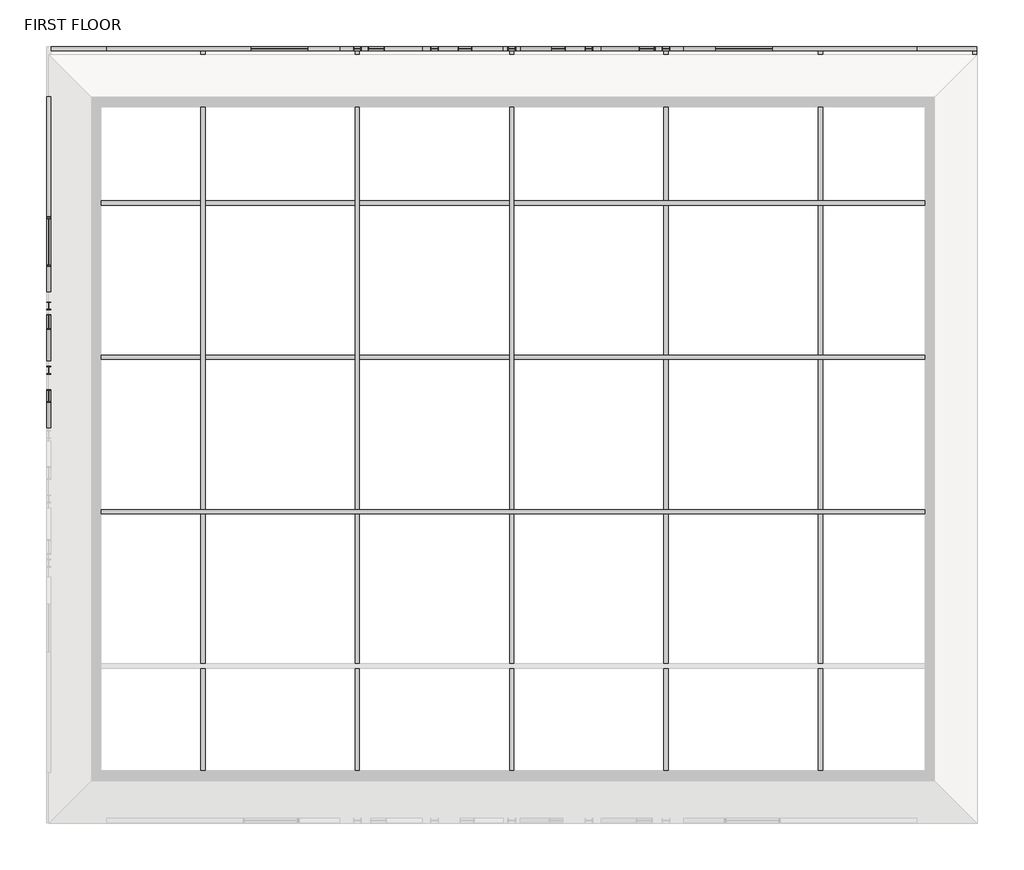
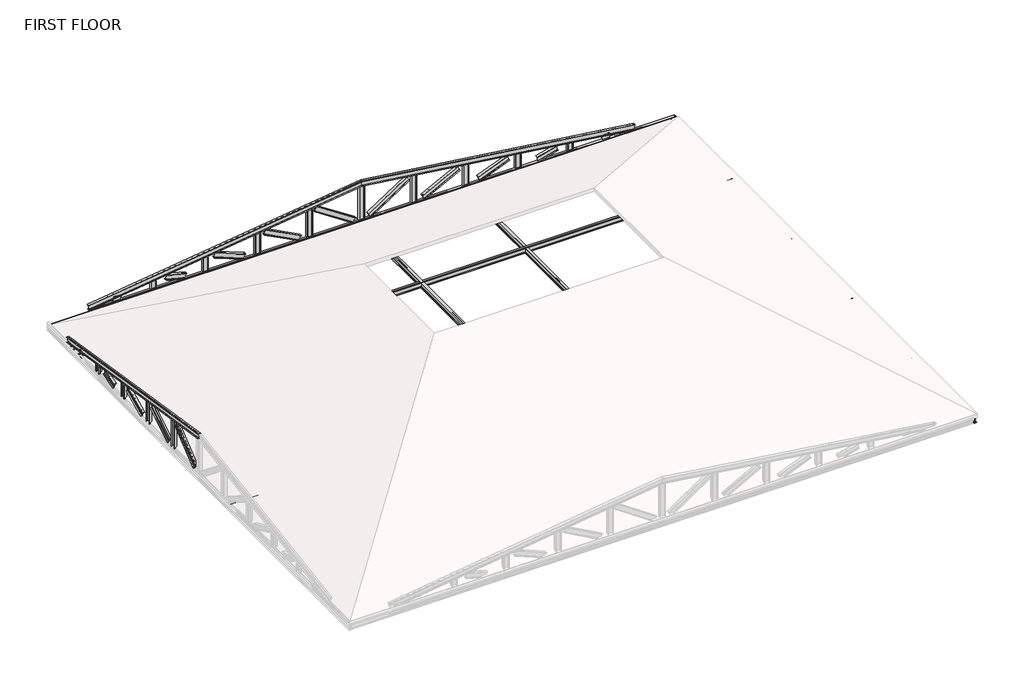
# One storey, part 2 of 2: 45 beams.
"""IFC4 building model written with IfcOpenShell, lengths in millimetres."""

from ifc_helpers import new_model, si_unit, frame, origin, place, context, project, spatial, polyline, circle_curve, ellipse_curve, transform, mapped, element, save
from ifc_brep_helpers import plane_surface, revolved_surface, advanced_brep
from components import ub_universal_beams_ub305x165x40_be890a2c, ub_universal_beams_ub305x165x40_a59d1a35, ub_universal_beams_ub305x165x40_0aabe8ba, ub_universal_beams_ub305x165x40_d04475ed, ub_universal_beams_ub305x165x40_f264fe8a, ub_universal_beams_ub305x165x40_2f8ff02f, ub_universal_beams_ub305x165x40_4bff7ce7, ub_universal_beams_ub305x165x40_d5ce0422, ub_universal_beams_ub305x165x40_0af343aa, ub_universal_beams_ub305x165x40_6c2df09e, ub_universal_beams_ub305x165x40_9aefeb6a, ub_universal_beams_ub305x165x40_8fd3c0bc, ub_universal_beams_ub305x165x40_dcb3c2ea, ub_universal_beams_ub305x165x40_5cbd381f, ub_universal_beams_ub305x165x40_28de461c, ub_universal_beams_ub305x165x40_2a071682, ub_universal_beams_ub305x165x40_a83b25bc, ub_universal_beams_ub305x165x40_c2ddfea9, ub_universal_beams_ub305x165x40_890a58b8, ub_universal_beams_ub305x165x40_8a566974, ub_universal_beams_ub305x165x40_7abb9ae2, ub_universal_beams_ub305x165x40_eb09afc0, ub_universal_beams_ub305x165x40_07ff8ca2, ub_universal_beams_ub305x165x40_bc9e57b7, ub_universal_beams_ub305x165x40_1f6689ec, ub_universal_beams_ub305x165x40_ea68f55e, ub_universal_beams_ub305x165x40_862170f4, ub_universal_beams_ub305x165x40_9b118c67, ub_universal_beams_ub305x165x40_fca44d3c, ub_universal_beams_ub305x165x40_5ea05da3

model = new_model("IFC4")

# Units and contexts
model_context = context("Model", 3, world=origin())
ifc_project = project(units=[si_unit("LENGTHUNIT", "METRE", prefix="MILLI")], contexts=[model_context])

# Site, building, storey
site = spatial("IfcSite", under=ifc_project)
building = spatial("IfcBuilding", under=site)
storey = spatial("IfcBuildingStorey", under=building, Name="FIRST FLOOR", Elevation=2454.6695361)

# Beams
placement = place(None, origin())
element("IfcBeam", 1, ObjectType="UB-Universal Beams : UB305x165x40", at=placement, inside=storey, context=model_context, shape_type="AdvancedBrep", body=[
    advanced_brep(
    [(-16297.3812503, 24370.7691735, 2618.146307), (-16296.0540475, 24370.7691735, 2608.033022), (-16296.0540475, 24205.7691735, 2608.033022), (-16297.3812503, 24205.7691735, 2618.146307), (-16297.3812503, 24276.3691735, 2618.146307), (-16298.5392997, 24285.2691735, 2626.9706439), (-16333.0465713, 24285.2691735, 2889.9160531), (-16334.2046207, 24276.3691735, 2898.7403899), (-16334.2046207, 24205.7691735, 2898.7403899), (-16335.5318235, 24205.7691735, 2908.8536749), (-16335.5318235, 24370.7691735, 2908.8536749), (-16334.2046207, 24370.7691735, 2898.7403899), (-16334.2046207, 24300.1691735, 2898.7403899), (-16333.0465713, 24291.2691735, 2889.9160531), (-16298.5392997, 24291.2691735, 2626.9706439), (-16297.3812503, 24300.1691735, 2618.146307), (-342.5493858, 24300.1691735, 4711.9562629), (-342.5493858, 24370.7691735, 4711.9562629), (-342.5493858, 24291.2691735, 4720.9325748), (-342.5493858, 24291.2691735, 4988.4064973), (-342.5493858, 24300.1691735, 4997.3828092), (-342.5493858, 24370.7691735, 4997.3828092), (-342.5493858, 24370.7691735, 5007.6702678), (-342.5493858, 24205.7691735, 5007.6702678), (-342.5493858, 24205.7691735, 4997.3828092), (-342.5493858, 24276.3691735, 4997.3828092), (-342.5493858, 24285.2691735, 4988.4064973), (-342.5493858, 24285.2691735, 4720.9325748), (-342.5493858, 24276.3691735, 4711.9562629), (-342.5493858, 24205.7691735, 4711.9562629), (-342.5493858, 24205.7691735, 4701.6688044), (-342.5493858, 24370.7691735, 4701.6688044)],
    [
        (0, 1),
        (1, 2),
        (2, 3),
        (3, 4),
        (4, 5, circle_curve(frame((-16298.5392997, 24276.3691735, 2626.9706439), z_axis=(0.9914985263311615, 0.0, 0.13011791684135987), x_axis=(0.0, -1.0, 0.0)), 8.9)),
        (5, 6),
        (6, 7, circle_curve(frame((-16333.0465713, 24276.3691735, 2889.9160531), z_axis=(0.9914985263311615, 0.0, 0.13011791684135987), x_axis=(0.0, -1.0, 0.0)), 8.9)),
        (7, 8),
        (8, 9),
        (9, 10),
        (10, 11),
        (11, 12),
        (12, 13, circle_curve(frame((-16333.0465713, 24300.1691735, 2889.9160531), z_axis=(0.9914985263311615, 0.0, 0.13011791684135987), x_axis=(0.0, -1.0, 0.0)), 8.9)),
        (13, 14),
        (14, 15, circle_curve(frame((-16298.5392997, 24300.1691735, 2626.9706439), z_axis=(0.9914985263311615, 0.0, 0.13011791684135987), x_axis=(0.0, -1.0, 0.0)), 8.9)),
        (15, 0),
        (16, 17),
        (17, 0),
        (15, 16),
        (18, 16, ellipse_curve(frame((-342.5493858, 24300.1691735, 4720.9325748), z_axis=(1.0, 0.0, 0.0), x_axis=(0.0, 0.0, -0.9999999999999999)), 8.9763119, 8.9)),
        (14, 18),
        (19, 18),
        (13, 19),
        (20, 19, ellipse_curve(frame((-342.5493858, 24300.1691735, 4988.4064973), z_axis=(1.0, 0.0, 0.0), x_axis=(0.0, 0.0, -0.9999999999999999)), 8.9763119, 8.9)),
        (12, 20),
        (21, 20),
        (11, 21),
        (22, 21),
        (10, 22),
        (23, 22),
        (9, 23),
        (24, 23),
        (8, 24),
        (25, 24),
        (7, 25),
        (26, 25, ellipse_curve(frame((-342.5493858, 24276.3691735, 4988.4064973), z_axis=(1.0, 0.0, 0.0), x_axis=(0.0, 0.0, -0.9999999999999999)), 8.9763119, 8.9)),
        (6, 26),
        (27, 26),
        (5, 27),
        (28, 27, ellipse_curve(frame((-342.5493858, 24276.3691735, 4720.9325748), z_axis=(1.0, 0.0, 0.0), x_axis=(0.0, 0.0, -0.9999999999999999)), 8.9763119, 8.9)),
        (4, 28),
        (29, 28),
        (3, 29),
        (30, 29),
        (2, 30),
        (31, 30),
        (1, 31),
        (17, 31),
    ],
    [
        plane_surface(frame((-16315.7929355, 24288.2691735, 2758.4433485), z_axis=(-0.9914985263311615, 0.0, -0.13011791684135987), x_axis=(-0.13011791684135987, 0.0, 0.9914985263311615))),
        plane_surface(frame((-324.1416914, 24370.7691735, 4714.3719709), z_axis=(-0.13011791684135987, 0.0, 0.9914985263311615), x_axis=(-0.9914985263311615, 0.0, -0.13011791684135987))),
        revolved_surface(polyline([(-16298.5392997612, 24291.269173499997, 2626.970643894329), (-341.39133634520147, 24291.269173499997, 4721.084549854435)]), (-325.2997408, 24300.1691735, 4723.1963078), (-0.9914985263311615, 0.0, -0.13011791684135987)),
        plane_surface(frame((-325.2997408, 24291.2691735, 4723.1963078), z_axis=(0.0, 1.0, 0.0), x_axis=(-0.9914985263311615, 0.0, -0.13011791684135987))),
        revolved_surface(polyline([(-16333.046571287405, 24291.269173499997, 2889.9160530040135), (-341.3913363366006, 24291.269173499997, 4988.558472288897)]), (-359.8070124, 24300.1691735, 4986.1417169), (-0.9914985263311615, 0.0, -0.13011791684135987)),
        plane_surface(frame((-360.9650618, 24300.1691735, 4994.9660538), z_axis=(0.13011791684135987, 0.0, -0.9914985263311615), x_axis=(-0.9914985263311615, 0.0, -0.13011791684135987))),
        plane_surface(frame((-360.9650618, 24370.7691735, 4994.9660538), z_axis=(0.0, 1.0, 0.0), x_axis=(-0.9914985263311615, 0.0, -0.13011791684135987))),
        plane_surface(frame((-362.2922646, 24370.7691735, 5005.0793388), z_axis=(-0.13011791684135987, 0.0, 0.9914985263311615), x_axis=(-0.9914985263311615, 0.0, -0.13011791684135987))),
        plane_surface(frame((-362.2922646, 24205.7691735, 5005.0793388), z_axis=(0.0, -1.0, 0.0), x_axis=(-0.9914985263311615, 0.0, -0.13011791684135987))),
        plane_surface(frame((-360.9650618, 24205.7691735, 4994.9660538), z_axis=(0.13011791684135987, 0.0, -0.9914985263311615), x_axis=(-0.9914985263311615, 0.0, -0.13011791684135987))),
        revolved_surface(polyline([(-16333.046571287405, 24267.469173499998, 2889.9160530040135), (-341.3913363366006, 24267.469173499998, 4988.558472288897)]), (-359.8070124, 24276.3691735, 4986.1417169), (-0.9914985263311615, 0.0, -0.13011791684135987)),
        plane_surface(frame((-359.8070124, 24285.2691735, 4986.1417169), z_axis=(0.0, -1.0, 0.0), x_axis=(-0.9914985263311615, 0.0, -0.13011791684135987))),
        revolved_surface(polyline([(-16298.5392997612, 24267.469173499998, 2626.970643894329), (-341.39133634520147, 24267.469173499998, 4721.084549854435)]), (-325.2997408, 24276.3691735, 4723.1963078), (-0.9914985263311615, 0.0, -0.13011791684135987)),
        plane_surface(frame((-324.1416914, 24276.3691735, 4714.3719709), z_axis=(-0.13011791684135987, 0.0, 0.9914985263311615), x_axis=(-0.9914985263311615, 0.0, -0.13011791684135987))),
        plane_surface(frame((-324.1416914, 24205.7691735, 4714.3719709), z_axis=(0.0, -1.0, 0.0), x_axis=(-0.9914985263311615, 0.0, -0.13011791684135987))),
        plane_surface(frame((-322.8144886, 24205.7691735, 4704.2586859), z_axis=(0.13011791684135987, 0.0, -0.9914985263311615), x_axis=(-0.9914985263311615, 0.0, -0.13011791684135987))),
        plane_surface(frame((-322.8144886, 24370.7691735, 4704.2586859), z_axis=(0.0, 1.0, 0.0), x_axis=(-0.9914985263311615, 0.0, -0.13011791684135987))),
        plane_surface(frame((-342.5493858, 24288.2691735, 5007.6702678), z_axis=(1.0, 0.0, 0.0), x_axis=(0.0, -1.0, 0.0))),
    ],
    [
        (0, [[1, 2, 3, 4, 5, 6, 7, 8, 9, 10, 11, 12, 13, 14, 15, 16]]),
        (1, [[17, 18, -16, 19]]),
        (2, [[20, -19, -15, 21]]),
        (3, [[22, -21, -14, 23]]),
        (4, [[24, -23, -13, 25]]),
        (5, [[26, -25, -12, 27]]),
        (6, [[28, -27, -11, 29]]),
        (7, [[30, -29, -10, 31]]),
        (8, [[32, -31, -9, 33]]),
        (9, [[34, -33, -8, 35]]),
        (10, [[36, -35, -7, 37]]),
        (11, [[38, -37, -6, 39]]),
        (12, [[40, -39, -5, 41]]),
        (13, [[42, -41, -4, 43]]),
        (14, [[44, -43, -3, 45]]),
        (15, [[46, -45, -2, 47]]),
        (16, [[48, -47, -1, -18]]),
        (17, [[-17, -20, -22, -24, -26, -28, -30, -32, -34, -36, -38, -40, -42, -44, -46, -48]]),
    ],
),
])
element("IfcBeam", 2, ObjectType="UB-Universal Beams : UB305x165x40", at=placement, inside=storey, context=model_context, shape_type="AdvancedBrep", body=[
    advanced_brep(
    [(15612.2824786, 24370.7691735, 2618.146307), (15612.2824786, 24300.1691735, 2618.146307), (15613.4405281, 24291.2691735, 2626.9706439), (15647.9477996, 24291.2691735, 2889.9160531), (15649.1058491, 24300.1691735, 2898.7403899), (15649.1058491, 24370.7691735, 2898.7403899), (15650.4330518, 24370.7691735, 2908.8536749), (15650.4330518, 24205.7691735, 2908.8536749), (15649.1058491, 24205.7691735, 2898.7403899), (15649.1058491, 24276.3691735, 2898.7403899), (15647.9477996, 24285.2691735, 2889.9160531), (15613.4405281, 24285.2691735, 2626.9706439), (15612.2824786, 24276.3691735, 2618.146307), (15612.2824786, 24205.7691735, 2618.146307), (15610.9552758, 24205.7691735, 2608.033022), (15610.9552758, 24370.7691735, 2608.033022), (-342.5493858, 24370.7691735, 4711.9562629), (-342.5493858, 24300.1691735, 4711.9562629), (-342.5493858, 24291.2691735, 4720.9325748), (-342.5493858, 24291.2691735, 4988.4064973), (-342.5493858, 24300.1691735, 4997.3828092), (-342.5493858, 24370.7691735, 4997.3828092), (-342.5493858, 24370.7691735, 5007.6702678), (-342.5493858, 24205.7691735, 5007.6702678), (-342.5493858, 24205.7691735, 4997.3828092), (-342.5493858, 24276.3691735, 4997.3828092), (-342.5493858, 24285.2691735, 4988.4064973), (-342.5493858, 24285.2691735, 4720.9325748), (-342.5493858, 24276.3691735, 4711.9562629), (-342.5493858, 24205.7691735, 4711.9562629), (-342.5493858, 24205.7691735, 4701.6688044), (-342.5493858, 24370.7691735, 4701.6688044)],
    [
        (0, 1),
        (1, 2, circle_curve(frame((15613.4405281, 24300.1691735, 2626.9706439), z_axis=(-0.9914985263311615, 0.0, 0.13011791684135987), x_axis=(0.0, -1.0, 0.0)), 8.9)),
        (2, 3),
        (3, 4, circle_curve(frame((15647.9477996, 24300.1691735, 2889.9160531), z_axis=(-0.9914985263311615, 0.0, 0.13011791684135987), x_axis=(0.0, -1.0, 0.0)), 8.9)),
        (4, 5),
        (5, 6),
        (6, 7),
        (7, 8),
        (8, 9),
        (9, 10, circle_curve(frame((15647.9477996, 24276.3691735, 2889.9160531), z_axis=(-0.9914985263311615, 0.0, 0.13011791684135987), x_axis=(0.0, -1.0, 0.0)), 8.9)),
        (10, 11),
        (11, 12, circle_curve(frame((15613.4405281, 24276.3691735, 2626.9706439), z_axis=(-0.9914985263311615, 0.0, 0.13011791684135987), x_axis=(0.0, -1.0, 0.0)), 8.9)),
        (12, 13),
        (13, 14),
        (14, 15),
        (15, 0),
        (0, 16),
        (16, 17),
        (17, 1),
        (17, 18, ellipse_curve(frame((-342.5493858, 24300.1691735, 4720.9325748), z_axis=(-1.0, 0.0, 0.0), x_axis=(0.0, 0.0, 1.0)), 8.9763119, 8.9)),
        (18, 2),
        (18, 19),
        (19, 3),
        (19, 20, ellipse_curve(frame((-342.5493858, 24300.1691735, 4988.4064973), z_axis=(-1.0, 0.0, 0.0), x_axis=(0.0, 0.0, 1.0)), 8.9763119, 8.9)),
        (20, 4),
        (20, 21),
        (21, 5),
        (21, 22),
        (22, 6),
        (22, 23),
        (23, 7),
        (23, 24),
        (24, 8),
        (24, 25),
        (25, 9),
        (25, 26, ellipse_curve(frame((-342.5493858, 24276.3691735, 4988.4064973), z_axis=(-1.0, 0.0, 0.0), x_axis=(0.0, 0.0, 1.0)), 8.9763119, 8.9)),
        (26, 10),
        (26, 27),
        (27, 11),
        (27, 28, ellipse_curve(frame((-342.5493858, 24276.3691735, 4720.9325748), z_axis=(-1.0, 0.0, 0.0), x_axis=(0.0, 0.0, 1.0)), 8.9763119, 8.9)),
        (28, 12),
        (28, 29),
        (29, 13),
        (29, 30),
        (30, 14),
        (30, 31),
        (31, 15),
        (31, 16),
    ],
    [
        plane_surface(frame((15630.6941638, 24288.2691735, 2758.4433485), z_axis=(0.9914985263311615, 0.0, -0.13011791684135987), x_axis=(0.13011791684135987, 0.0, 0.9914985263311615))),
        plane_surface(frame((15612.2824786, 24370.7691735, 2618.146307), z_axis=(0.13011791684135987, 0.0, 0.9914985263311615), x_axis=(-0.9914985263311615, 0.0, 0.13011791684135987))),
        revolved_surface(polyline([(-343.70743525510625, 24291.269173499997, 4721.084549852116), (15613.4405281, 24291.269173499997, 2626.9706439)]), (15613.4405281, 24300.1691735, 2626.9706439), (-0.9914985263311615, 0.0, 0.13011791684135987)),
        plane_surface(frame((15613.4405281, 24291.2691735, 2626.9706439), z_axis=(0.0, 1.0, 0.0), x_axis=(-0.9914985263311615, 0.0, 0.13011791684135987))),
        revolved_surface(polyline([(-343.707435252496, 24291.269173499997, 4988.558472371982), (15647.947799650316, 24291.269173499997, 2889.9160530933973)]), (15647.9477996, 24300.1691735, 2889.9160531), (-0.9914985263311615, 0.0, 0.13011791684135987)),
        plane_surface(frame((15649.1058491, 24300.1691735, 2898.7403899), z_axis=(-0.13011791684135987, 0.0, -0.9914985263311615), x_axis=(-0.9914985263311615, 0.0, 0.13011791684135987))),
        plane_surface(frame((15649.1058491, 24370.7691735, 2898.7403899), z_axis=(0.0, 1.0, 0.0), x_axis=(-0.9914985263311615, 0.0, 0.13011791684135987))),
        plane_surface(frame((15650.4330518, 24370.7691735, 2908.8536749), z_axis=(0.13011791684135987, 0.0, 0.9914985263311615), x_axis=(-0.9914985263311615, 0.0, 0.13011791684135987))),
        plane_surface(frame((15650.4330518, 24205.7691735, 2908.8536749), z_axis=(0.0, -1.0, 0.0), x_axis=(-0.9914985263311615, 0.0, 0.13011791684135987))),
        plane_surface(frame((15649.1058491, 24205.7691735, 2898.7403899), z_axis=(-0.13011791684135987, 0.0, -0.9914985263311615), x_axis=(-0.9914985263311615, 0.0, 0.13011791684135987))),
        revolved_surface(polyline([(-343.707435252496, 24267.469173499998, 4988.558472371982), (15647.947799650316, 24267.469173499998, 2889.9160530933973)]), (15647.9477996, 24276.3691735, 2889.9160531), (-0.9914985263311615, 0.0, 0.13011791684135987)),
        plane_surface(frame((15647.9477996, 24285.2691735, 2889.9160531), z_axis=(0.0, -1.0, 0.0), x_axis=(-0.9914985263311615, 0.0, 0.13011791684135987))),
        revolved_surface(polyline([(-343.70743525510625, 24267.469173499998, 4721.084549852116), (15613.4405281, 24267.469173499998, 2626.9706439)]), (15613.4405281, 24276.3691735, 2626.9706439), (-0.9914985263311615, 0.0, 0.13011791684135987)),
        plane_surface(frame((15612.2824786, 24276.3691735, 2618.146307), z_axis=(0.13011791684135987, 0.0, 0.9914985263311615), x_axis=(-0.9914985263311615, 0.0, 0.13011791684135987))),
        plane_surface(frame((15612.2824786, 24205.7691735, 2618.146307), z_axis=(0.0, -1.0, 0.0), x_axis=(-0.9914985263311615, 0.0, 0.13011791684135987))),
        plane_surface(frame((15610.9552758, 24205.7691735, 2608.033022), z_axis=(-0.13011791684135987, 0.0, -0.9914985263311615), x_axis=(-0.9914985263311615, 0.0, 0.13011791684135987))),
        plane_surface(frame((15610.9552758, 24370.7691735, 2608.033022), z_axis=(0.0, 1.0, 0.0), x_axis=(-0.9914985263311615, 0.0, 0.13011791684135987))),
        plane_surface(frame((-342.5493858, 24288.2691735, 5007.6702678), z_axis=(-1.0, 0.0, 0.0), x_axis=(0.0, 1.0, 0.0))),
    ],
    [
        (0, [[1, 2, 3, 4, 5, 6, 7, 8, 9, 10, 11, 12, 13, 14, 15, 16]]),
        (1, [[-1, 17, 18, 19]]),
        (2, [[-2, -19, 20, 21]]),
        (3, [[-3, -21, 22, 23]]),
        (4, [[-4, -23, 24, 25]]),
        (5, [[-5, -25, 26, 27]]),
        (6, [[-6, -27, 28, 29]]),
        (7, [[-7, -29, 30, 31]]),
        (8, [[-8, -31, 32, 33]]),
        (9, [[-9, -33, 34, 35]]),
        (10, [[-10, -35, 36, 37]]),
        (11, [[-11, -37, 38, 39]]),
        (12, [[-12, -39, 40, 41]]),
        (13, [[-13, -41, 42, 43]]),
        (14, [[-14, -43, 44, 45]]),
        (15, [[-15, -45, 46, 47]]),
        (16, [[-16, -47, 48, -17]]),
        (17, [[-48, -46, -44, -42, -40, -38, -36, -34, -32, -30, -28, -26, -24, -22, -20, -18]]),
    ],
),
])
element("IfcBeam", 3, ObjectType="UB-Universal Beams : UB305x165x40", at=placement, inside=storey, context=model_context, shape_type="AdvancedBrep", body=[
    advanced_brep(
    [(-18713.0493858, 22338.8015951, 2618.4284465), (-18642.4493858, 22338.8015951, 2618.4284465), (-18633.5493858, 22340.1861071, 2627.2200975), (-18633.5493858, 22381.4414523, 2889.1915396), (-18642.4493858, 22382.8259643, 2897.9831906), (-18713.0493858, 22382.8259643, 2897.9831906), (-18713.0493858, 22384.4127083, 2908.0590153), (-18548.0493858, 22384.4127083, 2908.0590153), (-18548.0493858, 22382.8259643, 2897.9831906), (-18618.6493858, 22382.8259643, 2897.9831906), (-18627.5493858, 22381.4414523, 2889.1915396), (-18627.5493858, 22340.1861071, 2627.2200975), (-18618.6493858, 22338.8015951, 2618.4284465), (-18548.0493858, 22338.8015951, 2618.4284465), (-18548.0493858, 22337.2148511, 2608.3526219), (-18713.0493858, 22337.2148511, 2608.3526219), (-18713.0493858, 9048.2691735, 4711.4256783), (-18642.4493858, 9048.2691735, 4711.4256783), (-18633.5493858, 9048.2691735, 4720.4353626), (-18633.5493858, 9048.2691735, 4988.9037095), (-18642.4493858, 9048.2691735, 4997.9133939), (-18713.0493858, 9048.2691735, 4997.9133939), (-18713.0493858, 9048.2691735, 5008.2390995), (-18548.0493858, 9048.2691735, 5008.2390995), (-18548.0493858, 9048.2691735, 4997.9133939), (-18618.6493858, 9048.2691735, 4997.9133939), (-18627.5493858, 9048.2691735, 4988.9037095), (-18627.5493858, 9048.2691735, 4720.4353626), (-18618.6493858, 9048.2691735, 4711.4256783), (-18548.0493858, 9048.2691735, 4711.4256783), (-18548.0493858, 9048.2691735, 4701.0999726), (-18713.0493858, 9048.2691735, 4701.0999726)],
    [
        (0, 1),
        (1, 2, circle_curve(frame((-18642.4493858, 22340.1861071, 2627.2200975), z_axis=(0.0, -0.9878259507117182, 0.15556314184436523), x_axis=(1.0, 0.0, 0.0)), 8.9)),
        (2, 3),
        (3, 4, circle_curve(frame((-18642.4493858, 22381.4414523, 2889.1915396), z_axis=(0.0, -0.9878259507117182, 0.15556314184436523), x_axis=(1.0, 0.0, 0.0)), 8.9)),
        (4, 5),
        (5, 6),
        (6, 7),
        (7, 8),
        (8, 9),
        (9, 10, circle_curve(frame((-18618.6493858, 22381.4414523, 2889.1915396), z_axis=(0.0, -0.9878259507117182, 0.15556314184436523), x_axis=(1.0, 0.0, 0.0)), 8.9)),
        (10, 11),
        (11, 12, circle_curve(frame((-18618.6493858, 22340.1861071, 2627.2200975), z_axis=(0.0, -0.9878259507117182, 0.15556314184436523), x_axis=(1.0, 0.0, 0.0)), 8.9)),
        (12, 13),
        (13, 14),
        (14, 15),
        (15, 0),
        (0, 16),
        (16, 17),
        (17, 1),
        (17, 18, ellipse_curve(frame((-18642.4493858, 9048.2691735, 4720.4353626), z_axis=(0.0, -1.0, 0.0), x_axis=(0.0, 0.0, 1.0)), 9.0096843, 8.9)),
        (18, 2),
        (18, 19),
        (19, 3),
        (19, 20, ellipse_curve(frame((-18642.4493858, 9048.2691735, 4988.9037095), z_axis=(0.0, -1.0, 0.0), x_axis=(0.0, 0.0, 1.0)), 9.0096843, 8.9)),
        (20, 4),
        (20, 21),
        (21, 5),
        (21, 22),
        (22, 6),
        (22, 23),
        (23, 7),
        (23, 24),
        (24, 8),
        (24, 25),
        (25, 9),
        (25, 26, ellipse_curve(frame((-18618.6493858, 9048.2691735, 4988.9037095), z_axis=(0.0, -1.0, 0.0), x_axis=(0.0, 0.0, 1.0)), 9.0096843, 8.9)),
        (26, 10),
        (26, 27),
        (27, 11),
        (27, 28, ellipse_curve(frame((-18618.6493858, 9048.2691735, 4720.4353626), z_axis=(0.0, -1.0, 0.0), x_axis=(0.0, 0.0, 1.0)), 9.0096843, 8.9)),
        (28, 12),
        (28, 29),
        (29, 13),
        (29, 30),
        (30, 14),
        (30, 31),
        (31, 15),
        (31, 16),
    ],
    [
        plane_surface(frame((-18630.5493858, 22360.8137797, 2758.2058186), z_axis=(0.0, 0.9878259507117182, -0.15556314184436523), x_axis=(0.0, 0.15556314184436523, 0.9878259507117182))),
        plane_surface(frame((-18713.0493858, 22338.8015951, 2618.4284465), z_axis=(0.0, 0.15556314184436523, 0.9878259507117182), x_axis=(0.0, -0.9878259507117182, 0.15556314184436523))),
        revolved_surface(polyline([(-18633.549385799997, 9046.884661549127, 4720.6533960119505), (-18633.549385799997, 22340.1861071, 2627.2200975)]), (-18642.4493858, 22340.1861071, 2627.2200975), (0.0, -0.9878259507117182, 0.15556314184436523)),
        plane_surface(frame((-18633.5493858, 22340.1861071, 2627.2200975), z_axis=(-1.0, 0.0, 0.0), x_axis=(0.0, -0.9878259507117182, 0.15556314184436523))),
        revolved_surface(polyline([(-18633.549385799997, 9046.884661526983, 4989.1217428713435), (-18633.549385799997, 22381.44145233073, 2889.1915395951605)]), (-18642.4493858, 22381.4414523, 2889.1915396), (0.0, -0.9878259507117182, 0.15556314184436523)),
        plane_surface(frame((-18642.4493858, 22382.8259643, 2897.9831906), z_axis=(0.0, -0.15556314184436523, -0.9878259507117182), x_axis=(0.0, -0.9878259507117182, 0.15556314184436523))),
        plane_surface(frame((-18713.0493858, 22382.8259643, 2897.9831906), z_axis=(-1.0, 0.0, 0.0), x_axis=(0.0, -0.9878259507117182, 0.15556314184436523))),
        plane_surface(frame((-18713.0493858, 22384.4127083, 2908.0590153), z_axis=(0.0, 0.15556314184436523, 0.9878259507117182), x_axis=(0.0, -0.9878259507117182, 0.15556314184436523))),
        plane_surface(frame((-18548.0493858, 22384.4127083, 2908.0590153), z_axis=(1.0, 0.0, 0.0), x_axis=(0.0, -0.9878259507117182, 0.15556314184436523))),
        plane_surface(frame((-18548.0493858, 22382.8259643, 2897.9831906), z_axis=(0.0, -0.15556314184436523, -0.9878259507117182), x_axis=(0.0, -0.9878259507117182, 0.15556314184436523))),
        revolved_surface(polyline([(-18609.749385799998, 9046.884661526983, 4989.1217428713435), (-18609.749385799998, 22381.44145233073, 2889.1915395951605)]), (-18618.6493858, 22381.4414523, 2889.1915396), (0.0, -0.9878259507117182, 0.15556314184436523)),
        plane_surface(frame((-18627.5493858, 22381.4414523, 2889.1915396), z_axis=(1.0, 0.0, 0.0), x_axis=(0.0, -0.9878259507117182, 0.15556314184436523))),
        revolved_surface(polyline([(-18609.749385799998, 9046.884661549127, 4720.6533960119505), (-18609.749385799998, 22340.1861071, 2627.2200975)]), (-18618.6493858, 22340.1861071, 2627.2200975), (0.0, -0.9878259507117182, 0.15556314184436523)),
        plane_surface(frame((-18618.6493858, 22338.8015951, 2618.4284465), z_axis=(0.0, 0.15556314184436523, 0.9878259507117182), x_axis=(0.0, -0.9878259507117182, 0.15556314184436523))),
        plane_surface(frame((-18548.0493858, 22338.8015951, 2618.4284465), z_axis=(1.0, 0.0, 0.0), x_axis=(0.0, -0.9878259507117182, 0.15556314184436523))),
        plane_surface(frame((-18548.0493858, 22337.2148511, 2608.3526219), z_axis=(0.0, -0.15556314184436523, -0.9878259507117182), x_axis=(0.0, -0.9878259507117182, 0.15556314184436523))),
        plane_surface(frame((-18713.0493858, 22337.2148511, 2608.3526219), z_axis=(-1.0, 0.0, 0.0), x_axis=(0.0, -0.9878259507117182, 0.15556314184436523))),
        plane_surface(frame((-18630.5493858, 9048.2691735, 5008.2390995), z_axis=(0.0, -1.0, 0.0), x_axis=(0.0, 0.0, 1.0))),
    ],
    [
        (0, [[1, 2, 3, 4, 5, 6, 7, 8, 9, 10, 11, 12, 13, 14, 15, 16]]),
        (1, [[-1, 17, 18, 19]]),
        (2, [[-2, -19, 20, 21]]),
        (3, [[-3, -21, 22, 23]]),
        (4, [[-4, -23, 24, 25]]),
        (5, [[-5, -25, 26, 27]]),
        (6, [[-6, -27, 28, 29]]),
        (7, [[-7, -29, 30, 31]]),
        (8, [[-8, -31, 32, 33]]),
        (9, [[-9, -33, 34, 35]]),
        (10, [[-10, -35, 36, 37]]),
        (11, [[-11, -37, 38, 39]]),
        (12, [[-12, -39, 40, 41]]),
        (13, [[-13, -41, 42, 43]]),
        (14, [[-14, -43, 44, 45]]),
        (15, [[-15, -45, 46, 47]]),
        (16, [[-16, -47, 48, -17]]),
        (17, [[-48, -46, -44, -42, -40, -38, -36, -34, -32, -30, -28, -26, -24, -22, -20, -18]]),
    ],
),
])
ub_universal_beams_ub305x165x40_shape = ub_universal_beams_ub305x165x40_be890a2c(model_context)
element("IfcBeam", 4, ObjectType="UB-Universal Beams : UB305x165x40", at=placement, inside=storey, context=model_context, shape_type="MappedRepresentation", body=[
    mapped(ub_universal_beams_ub305x165x40_shape, transform((-12534.5493858, 9048.2691735, 2302.9695361), x_axis=(0.0, -1.0, 0.0), y_axis=(1.0, 0.0, 0.0), z_axis=(0.0, 0.0, 1.0))),
])
element("IfcBeam", 5, ObjectType="UB-Universal Beams : UB305x165x40", at=placement, inside=storey, context=model_context, shape_type="MappedRepresentation", body=[
    mapped(ub_universal_beams_ub305x165x40_shape, transform((-6438.5493858, 9048.2691735, 2302.9695361), x_axis=(0.0, -1.0, 0.0), y_axis=(1.0, 0.0, 0.0), z_axis=(0.0, 0.0, 1.0))),
])
element("IfcBeam", 6, ObjectType="UB-Universal Beams : UB305x165x40", at=placement, inside=storey, context=model_context, shape_type="MappedRepresentation", body=[
    mapped(ub_universal_beams_ub305x165x40_shape, transform((-342.5493858, 9048.2691735, 2302.9695361), x_axis=(0.0, -1.0, 0.0), y_axis=(1.0, 0.0, 0.0), z_axis=(0.0, 0.0, 1.0))),
])
element("IfcBeam", 7, ObjectType="UB-Universal Beams : UB305x165x40", at=placement, inside=storey, context=model_context, shape_type="MappedRepresentation", body=[
    mapped(ub_universal_beams_ub305x165x40_shape, transform((5753.4506142, 9048.2691735, 2302.9695361), x_axis=(0.0, -1.0, 0.0), y_axis=(1.0, 0.0, 0.0), z_axis=(0.0, 0.0, 1.0))),
])
element("IfcBeam", 8, ObjectType="UB-Universal Beams : UB305x165x40", at=placement, inside=storey, context=model_context, shape_type="MappedRepresentation", body=[
    mapped(ub_universal_beams_ub305x165x40_shape, transform((11849.4506142, 9048.2691735, 2302.9695361), x_axis=(0.0, -1.0, 0.0), y_axis=(1.0, 0.0, 0.0), z_axis=(0.0, 0.0, 1.0))),
])
ub_universal_beams_ub305x165x40_2_shape = ub_universal_beams_ub305x165x40_a59d1a35(model_context)
element("IfcBeam", 9, ObjectType="UB-Universal Beams : UB305x165x40", at=placement, inside=storey, context=model_context, shape_type="MappedRepresentation", body=[
    mapped(ub_universal_beams_ub305x165x40_2_shape, transform((-342.5493858, 24288.2691735, 2302.9695361), x_axis=(1.0, 0.0, 0.0), y_axis=(0.0, 1.0, 0.0), z_axis=(0.0, 0.0, 1.0))),
])
element("IfcBeam", 10, ObjectType="UB-Universal Beams : UB305x165x40", at=placement, inside=storey, context=model_context, shape_type="MappedRepresentation", body=[
    mapped(ub_universal_beams_ub305x165x40_2_shape, transform((-342.5493858, 18192.2691735, 2302.9695361), x_axis=(1.0, 0.0, 0.0), y_axis=(0.0, 1.0, 0.0), z_axis=(0.0, 0.0, 1.0))),
])
element("IfcBeam", 11, ObjectType="UB-Universal Beams : UB305x165x40", at=placement, inside=storey, context=model_context, shape_type="MappedRepresentation", body=[
    mapped(ub_universal_beams_ub305x165x40_2_shape, transform((-342.5493858, 12096.2691735, 2302.9695361), x_axis=(1.0, 0.0, 0.0), y_axis=(0.0, 1.0, 0.0), z_axis=(0.0, 0.0, 1.0))),
])
element("IfcBeam", 12, ObjectType="UB-Universal Beams : UB305x165x40", at=placement, inside=storey, context=model_context, shape_type="MappedRepresentation", body=[
    mapped(ub_universal_beams_ub305x165x40_2_shape, transform((-342.5493858, 6000.2691735, 2302.9695361), x_axis=(1.0, 0.0, 0.0), y_axis=(0.0, 1.0, 0.0), z_axis=(0.0, 0.0, 1.0))),
])
ub_universal_beams_ub305x165x40_3_shape = ub_universal_beams_ub305x165x40_0aabe8ba(model_context)
element("IfcBeam", 13, ObjectType="UB-Universal Beams : UB305x165x40", at=placement, inside=storey, context=model_context, shape_type="MappedRepresentation", body=[
    mapped(ub_universal_beams_ub305x165x40_3_shape, transform((17945.4506142, 9048.2691735, 2302.9695361), x_axis=(0.0, -1.0, 0.0), y_axis=(1.0, 0.0, 0.0), z_axis=(0.0, 0.0, 1.0))),
])
ub_universal_beams_ub305x165x40_4_shape = ub_universal_beams_ub305x165x40_d04475ed(model_context)
element("IfcBeam", 14, ObjectType="UB-Universal Beams : UB305x165x40", at=placement, inside=storey, context=model_context, shape_type="MappedRepresentation", body=[
    mapped(ub_universal_beams_ub305x165x40_4_shape, transform((-342.5493858, 24288.2691735, 3654.6695361), x_axis=(0.0, 0.0, 1.0), y_axis=(0.0, -1.0, 0.0), z_axis=(1.0, 0.0, 0.0))),
])
ub_universal_beams_ub305x165x40_5_shape = ub_universal_beams_ub305x165x40_f264fe8a(model_context)
element("IfcBeam", 15, ObjectType="UB-Universal Beams : UB305x165x40", at=placement, inside=storey, context=model_context, shape_type="MappedRepresentation", body=[
    mapped(ub_universal_beams_ub305x165x40_5_shape, transform((-3390.5493858, 24288.2691735, 3454.6695361), x_axis=(0.0, 0.0, 1.0), y_axis=(0.0, -1.0, 0.0), z_axis=(1.0, 0.0, 0.0))),
])
element("IfcBeam", 16, ObjectType="UB-Universal Beams : UB305x165x40", at=placement, inside=storey, context=model_context, shape_type="MappedRepresentation", body=[
    mapped(ub_universal_beams_ub305x165x40_5_shape, transform((2705.4506142, 24288.2691735, 3454.6695361), x_axis=(0.0, 0.0, 1.0), y_axis=(0.0, -1.0, 0.0), z_axis=(1.0, 0.0, 0.0))),
])
ub_universal_beams_ub305x165x40_6_shape = ub_universal_beams_ub305x165x40_2f8ff02f(model_context)
element("IfcBeam", 17, ObjectType="UB-Universal Beams : UB305x165x40", at=placement, inside=storey, context=model_context, shape_type="MappedRepresentation", body=[
    mapped(ub_universal_beams_ub305x165x40_6_shape, transform((-6438.5493858, 24288.2691735, 3254.6695361), x_axis=(0.0, 0.0, 1.0), y_axis=(0.0, -1.0, 0.0), z_axis=(1.0, 0.0, 0.0))),
])
element("IfcBeam", 18, ObjectType="UB-Universal Beams : UB305x165x40", at=placement, inside=storey, context=model_context, shape_type="MappedRepresentation", body=[
    mapped(ub_universal_beams_ub305x165x40_6_shape, transform((5753.4506142, 24288.2691735, 3254.6695361), x_axis=(0.0, 0.0, 1.0), y_axis=(0.0, -1.0, 0.0), z_axis=(1.0, 0.0, 0.0))),
])
ub_universal_beams_ub305x165x40_7_shape = ub_universal_beams_ub305x165x40_4bff7ce7(model_context)
element("IfcBeam", 19, ObjectType="UB-Universal Beams : UB305x165x40", at=placement, inside=storey, context=model_context, shape_type="MappedRepresentation", body=[
    mapped(ub_universal_beams_ub305x165x40_7_shape, transform((-9486.5493858, 24288.2691735, 3054.6695361), x_axis=(0.0, 0.0, 1.0), y_axis=(0.0, -1.0, 0.0), z_axis=(1.0, 0.0, 0.0))),
])
element("IfcBeam", 20, ObjectType="UB-Universal Beams : UB305x165x40", at=placement, inside=storey, context=model_context, shape_type="MappedRepresentation", body=[
    mapped(ub_universal_beams_ub305x165x40_7_shape, transform((8801.4506142, 24288.2691735, 3054.6695361), x_axis=(0.0, 0.0, 1.0), y_axis=(0.0, -1.0, 0.0), z_axis=(1.0, 0.0, 0.0))),
])
ub_universal_beams_ub305x165x40_8_shape = ub_universal_beams_ub305x165x40_d5ce0422(model_context)
element("IfcBeam", 21, ObjectType="UB-Universal Beams : UB305x165x40", at=placement, inside=storey, context=model_context, shape_type="MappedRepresentation", body=[
    mapped(ub_universal_beams_ub305x165x40_8_shape, transform((-12534.5493858, 24288.2691735, 2854.6695361), x_axis=(0.0, 0.0, 1.0), y_axis=(0.0, -1.0, 0.0), z_axis=(1.0, 0.0, 0.0))),
])
element("IfcBeam", 22, ObjectType="UB-Universal Beams : UB305x165x40", at=placement, inside=storey, context=model_context, shape_type="MappedRepresentation", body=[
    mapped(ub_universal_beams_ub305x165x40_8_shape, transform((11849.4506142, 24288.2691735, 2854.6695361), x_axis=(0.0, 0.0, 1.0), y_axis=(0.0, -1.0, 0.0), z_axis=(1.0, 0.0, 0.0))),
])
ub_universal_beams_ub305x165x40_9_shape = ub_universal_beams_ub305x165x40_0af343aa(model_context)
element("IfcBeam", 23, ObjectType="UB-Universal Beams : UB305x165x40", at=placement, inside=storey, context=model_context, shape_type="MappedRepresentation", body=[
    mapped(ub_universal_beams_ub305x165x40_9_shape, transform((-15582.5493858, 24288.2691735, 2654.6695361), x_axis=(0.0, 0.0, 1.0), y_axis=(0.0, -1.0, 0.0), z_axis=(1.0, 0.0, 0.0))),
])
element("IfcBeam", 24, ObjectType="UB-Universal Beams : UB305x165x40", at=placement, inside=storey, context=model_context, shape_type="MappedRepresentation", body=[
    mapped(ub_universal_beams_ub305x165x40_9_shape, transform((14897.4506142, 24288.2691735, 2654.6695361), x_axis=(0.0, 0.0, 1.0), y_axis=(0.0, -1.0, 0.0), z_axis=(1.0, 0.0, 0.0))),
])
ub_universal_beams_ub305x165x40_10_shape = ub_universal_beams_ub305x165x40_6c2df09e(model_context)
element("IfcBeam", 25, ObjectType="UB-Universal Beams : UB305x165x40", at=placement, inside=storey, context=model_context, shape_type="MappedRepresentation", body=[
    mapped(ub_universal_beams_ub305x165x40_10_shape, transform((-1866.5493858, 24288.2691735, 3454.6695361), x_axis=(0.8360793655139381, 0.0, -0.5486085075550785), y_axis=(0.0, -1.0, 0.0), z_axis=(-0.5486085075550785, 0.0, -0.8360793655139381))),
])
ub_universal_beams_ub305x165x40_11_shape = ub_universal_beams_ub305x165x40_9aefeb6a(model_context)
element("IfcBeam", 26, ObjectType="UB-Universal Beams : UB305x165x40", at=placement, inside=storey, context=model_context, shape_type="MappedRepresentation", body=[
    mapped(ub_universal_beams_ub305x165x40_11_shape, transform((-4914.5493858, 24288.2691735, 3254.6695361), x_axis=(0.8854218128752761, 0.0, -0.4647883532153745), y_axis=(0.0, -1.0, 0.0), z_axis=(-0.4647883532153745, 0.0, -0.8854218128752761))),
])
ub_universal_beams_ub305x165x40_12_shape = ub_universal_beams_ub305x165x40_8fd3c0bc(model_context)
element("IfcBeam", 27, ObjectType="UB-Universal Beams : UB305x165x40", at=placement, inside=storey, context=model_context, shape_type="MappedRepresentation", body=[
    mapped(ub_universal_beams_ub305x165x40_12_shape, transform((1181.4506142, 24288.2691735, 3454.6695361), x_axis=(0.8360793655139369, 0.0, 0.5486085075550804), y_axis=(0.0, -1.0, 0.0), z_axis=(0.5486085075550804, 0.0, -0.8360793655139369))),
])
ub_universal_beams_ub305x165x40_13_shape = ub_universal_beams_ub305x165x40_dcb3c2ea(model_context)
element("IfcBeam", 28, ObjectType="UB-Universal Beams : UB305x165x40", at=placement, inside=storey, context=model_context, shape_type="MappedRepresentation", body=[
    mapped(ub_universal_beams_ub305x165x40_13_shape, transform((4229.4506142, 24288.2691735, 3254.6695361), x_axis=(0.8854218128752784, 0.0, 0.46478835321537), y_axis=(0.0, -1.0, 0.0), z_axis=(0.46478835321537, 0.0, -0.8854218128752784))),
])
ub_universal_beams_ub305x165x40_14_shape = ub_universal_beams_ub305x165x40_5cbd381f(model_context)
element("IfcBeam", 29, ObjectType="UB-Universal Beams : UB305x165x40", at=placement, inside=storey, context=model_context, shape_type="MappedRepresentation", body=[
    mapped(ub_universal_beams_ub305x165x40_14_shape, transform((-7962.5493858, 24288.2691735, 3054.6695361), x_axis=(0.9304840855280709, 0.0, -0.36633231713703546), y_axis=(0.0, -1.0, 0.0), z_axis=(-0.36633231713703546, 0.0, -0.9304840855280709))),
])
ub_universal_beams_ub305x165x40_15_shape = ub_universal_beams_ub305x165x40_28de461c(model_context)
element("IfcBeam", 30, ObjectType="UB-Universal Beams : UB305x165x40", at=placement, inside=storey, context=model_context, shape_type="MappedRepresentation", body=[
    mapped(ub_universal_beams_ub305x165x40_15_shape, transform((7277.4506142, 24288.2691735, 3054.6695361), x_axis=(0.9304840855280697, 0.0, 0.36633231713703873), y_axis=(0.0, -1.0, 0.0), z_axis=(0.36633231713703873, 0.0, -0.9304840855280697))),
])
ub_universal_beams_ub305x165x40_16_shape = ub_universal_beams_ub305x165x40_2a071682(model_context)
element("IfcBeam", 31, ObjectType="UB-Universal Beams : UB305x165x40", at=placement, inside=storey, context=model_context, shape_type="MappedRepresentation", body=[
    mapped(ub_universal_beams_ub305x165x40_16_shape, transform((-11010.5493858, 24288.2691735, 2854.6695361), x_axis=(0.9672387579909856, 0.0, -0.2538684404175824), y_axis=(0.0, -1.0, 0.0), z_axis=(-0.2538684404175824, 0.0, -0.9672387579909856))),
])
ub_universal_beams_ub305x165x40_17_shape = ub_universal_beams_ub305x165x40_a83b25bc(model_context)
element("IfcBeam", 32, ObjectType="UB-Universal Beams : UB305x165x40", at=placement, inside=storey, context=model_context, shape_type="MappedRepresentation", body=[
    mapped(ub_universal_beams_ub305x165x40_17_shape, transform((10325.4506142, 24288.2691735, 2854.6695361), x_axis=(0.9672387579909859, 0.0, 0.2538684404175812), y_axis=(0.0, -1.0, 0.0), z_axis=(0.2538684404175812, 0.0, -0.9672387579909859))),
])
ub_universal_beams_ub305x165x40_18_shape = ub_universal_beams_ub305x165x40_c2ddfea9(model_context)
element("IfcBeam", 33, ObjectType="UB-Universal Beams : UB305x165x40", at=placement, inside=storey, context=model_context, shape_type="MappedRepresentation", body=[
    mapped(ub_universal_beams_ub305x165x40_18_shape, transform((13373.4506142, 24288.2691735, 2654.6695361), x_axis=(0.9914985263311615, 0.0, 0.1301179168413594), y_axis=(0.0, -1.0, 0.0), z_axis=(0.1301179168413594, 0.0, -0.9914985263311615))),
])
ub_universal_beams_ub305x165x40_19_shape = ub_universal_beams_ub305x165x40_890a58b8(model_context)
element("IfcBeam", 34, ObjectType="UB-Universal Beams : UB305x165x40", at=placement, inside=storey, context=model_context, shape_type="MappedRepresentation", body=[
    mapped(ub_universal_beams_ub305x165x40_19_shape, transform((-14058.5493858, 24288.2691735, 2654.6695361), x_axis=(0.9914985263311615, 0.0, -0.13011791684135912), y_axis=(0.0, -1.0, 0.0), z_axis=(-0.13011791684135912, 0.0, -0.9914985263311615))),
])
ub_universal_beams_ub305x165x40_20_shape = ub_universal_beams_ub305x165x40_8a566974(model_context)
element("IfcBeam", 35, ObjectType="UB-Universal Beams : UB305x165x40", at=placement, inside=storey, context=model_context, shape_type="MappedRepresentation", body=[
    mapped(ub_universal_beams_ub305x165x40_20_shape, transform((-18630.5493858, 11588.2691735, 3454.6695361), x_axis=(0.0, 0.0, 1.0), y_axis=(1.0, 0.0, 0.0), z_axis=(0.0, 1.0, 0.0))),
])
ub_universal_beams_ub305x165x40_21_shape = ub_universal_beams_ub305x165x40_7abb9ae2(model_context)
element("IfcBeam", 36, ObjectType="UB-Universal Beams : UB305x165x40", at=placement, inside=storey, context=model_context, shape_type="MappedRepresentation", body=[
    mapped(ub_universal_beams_ub305x165x40_21_shape, transform((-18630.5493858, 14128.2691735, 3254.6695361), x_axis=(0.0, 0.0, 1.0), y_axis=(1.0, 0.0, 0.0), z_axis=(0.0, 1.0, 0.0))),
])
ub_universal_beams_ub305x165x40_22_shape = ub_universal_beams_ub305x165x40_eb09afc0(model_context)
element("IfcBeam", 37, ObjectType="UB-Universal Beams : UB305x165x40", at=placement, inside=storey, context=model_context, shape_type="MappedRepresentation", body=[
    mapped(ub_universal_beams_ub305x165x40_22_shape, transform((-18630.5493858, 16668.2691735, 3054.6695361), x_axis=(0.0, 0.0, 1.0), y_axis=(1.0, 0.0, 0.0), z_axis=(0.0, 1.0, 0.0))),
])
ub_universal_beams_ub305x165x40_23_shape = ub_universal_beams_ub305x165x40_07ff8ca2(model_context)
element("IfcBeam", 38, ObjectType="UB-Universal Beams : UB305x165x40", at=placement, inside=storey, context=model_context, shape_type="MappedRepresentation", body=[
    mapped(ub_universal_beams_ub305x165x40_23_shape, transform((-18630.5493858, 19208.2691735, 2854.6695361), x_axis=(0.0, 0.0, 1.0), y_axis=(1.0, 0.0, 0.0), z_axis=(0.0, 1.0, 0.0))),
])
ub_universal_beams_ub305x165x40_24_shape = ub_universal_beams_ub305x165x40_bc9e57b7(model_context)
element("IfcBeam", 39, ObjectType="UB-Universal Beams : UB305x165x40", at=placement, inside=storey, context=model_context, shape_type="MappedRepresentation", body=[
    mapped(ub_universal_beams_ub305x165x40_24_shape, transform((-18630.5493858, 21748.2691735, 2654.6695361), x_axis=(0.0, 0.0, 1.0), y_axis=(1.0, 0.0, 0.0), z_axis=(0.0, 1.0, 0.0))),
])
ub_universal_beams_ub305x165x40_25_shape = ub_universal_beams_ub305x165x40_1f6689ec(model_context)
element("IfcBeam", 40, ObjectType="UB-Universal Beams : UB305x165x40", at=placement, inside=storey, context=model_context, shape_type="MappedRepresentation", body=[
    mapped(ub_universal_beams_ub305x165x40_25_shape, transform((-18630.5493858, 10318.2691735, 3454.6695361), x_axis=(0.0, 0.7856739006278272, 0.6186408666360921), y_axis=(1.0, 0.0, 0.0), z_axis=(0.0, 0.6186408666360921, -0.7856739006278272))),
])
ub_universal_beams_ub305x165x40_26_shape = ub_universal_beams_ub305x165x40_ea68f55e(model_context)
element("IfcBeam", 41, ObjectType="UB-Universal Beams : UB305x165x40", at=placement, inside=storey, context=model_context, shape_type="MappedRepresentation", body=[
    mapped(ub_universal_beams_ub305x165x40_26_shape, transform((-18630.5493858, 12858.2691735, 3254.6695361), x_axis=(0.0, 0.846121563913139, 0.5329899615200872), y_axis=(1.0, 0.0, 0.0), z_axis=(0.0, 0.5329899615200872, -0.846121563913139))),
])
ub_universal_beams_ub305x165x40_27_shape = ub_universal_beams_ub305x165x40_862170f4(model_context)
element("IfcBeam", 42, ObjectType="UB-Universal Beams : UB305x165x40", at=placement, inside=storey, context=model_context, shape_type="MappedRepresentation", body=[
    mapped(ub_universal_beams_ub305x165x40_27_shape, transform((-18630.5493858, 15398.2691735, 3054.6695361), x_axis=(0.0, 0.9041722720767187, 0.4271680025559315), y_axis=(1.0, 0.0, 0.0), z_axis=(0.0, 0.4271680025559315, -0.9041722720767187))),
])
ub_universal_beams_ub305x165x40_28_shape = ub_universal_beams_ub305x165x40_9b118c67(model_context)
element("IfcBeam", 43, ObjectType="UB-Universal Beams : UB305x165x40", at=placement, inside=storey, context=model_context, shape_type="MappedRepresentation", body=[
    mapped(ub_universal_beams_ub305x165x40_28_shape, transform((-18630.5493858, 17938.2691735, 2854.6695361), x_axis=(0.0, 0.9538094060666068, 0.30041241135956187), y_axis=(1.0, 0.0, 0.0), z_axis=(0.0, 0.30041241135956187, -0.9538094060666068))),
])
ub_universal_beams_ub305x165x40_29_shape = ub_universal_beams_ub305x165x40_fca44d3c(model_context)
element("IfcBeam", 44, ObjectType="UB-Universal Beams : UB305x165x40", at=placement, inside=storey, context=model_context, shape_type="MappedRepresentation", body=[
    mapped(ub_universal_beams_ub305x165x40_29_shape, transform((-18630.5493858, 20478.2691735, 2654.6695361), x_axis=(0.0, 0.9878259507117182, 0.1555631418443646), y_axis=(1.0, 0.0, 0.0), z_axis=(0.0, 0.1555631418443646, -0.9878259507117182))),
])
ub_universal_beams_ub305x165x40_30_shape = ub_universal_beams_ub305x165x40_5ea05da3(model_context)
element("IfcBeam", 45, ObjectType="UB-Universal Beams : UB305x165x40", at=placement, inside=storey, context=model_context, shape_type="MappedRepresentation", body=[
    mapped(ub_universal_beams_ub305x165x40_30_shape, transform((-342.5493858, 24288.2691735, 2454.6695361), x_axis=(1.0, 0.0, 0.0), y_axis=(0.0, 1.0, 0.0), z_axis=(0.0, 0.0, 1.0))),
])

save(model, "model.ifc")

# Revit data of these elements
# Type "UB-Universal Beams : UB305x165x40"
#   Section Name Key = "UB305X165X40"
#   Width = 16.5 cm
#   Web Thickness = 0.6 cm
#   Web Fillet = 0.89 cm
#   Warping Constant = 164000.0 cm⁶
#   Torsional Moment of Inertia = 14.70 cm⁴
#   Section Area = 51.3 cm²
#   Plastic Modulus weak axis = 142.0 cm³
#   Plastic Modulus strong axis = 623.0 cm³
#   Nominal Weight = 40.2999 kgf/m
#   Moment of Inertia weak axis = 764.00 cm⁴
#   Moment of Inertia strong axis = 8503.00 cm⁴
#   Height = 30.34 cm
#   Flange Thickness = 1.02 cm
#   Elastic Modulus weak axis = 92.6 cm³
#   Elastic Modulus strong axis = 560.0 cm³
#   Centroid Vertical = 15.17 cm
#   Centroid Horizontal = 8.25 cm
#   Bolt Spacing = 9.0 cm
#   Length [instance default] = 1500 mm
#   Structural Material [instance default] = Metal - Steel 43-275
#   Type Comments = ""
#   Assembly Code = ""
# Elements 1, 2, 3, 4, 5, 6, 7, 8, 9, 10, 11, 12, 13, 14, 15, 16, 17, 18, 19, 20, 21, 22, 23, 24, 25, 26, 27, 28, 29, 30, 31, 32, 33, 34, 35, 36, 37, 38, 39, 40, 41, 42, 43, 44, 45 (IfcBeam, "UB-Universal Beams : UB305x165x40")
#   Structural Material = Metal - Steel 43-275
#   Phase Created = New Construction
#   Materials on its faces: "Metal - Steel 43-275"
# Materials
#   "Metal - Steel 43-275": class "Metal", colour RGB 247 247 247, transparency 0, Cost = 0
